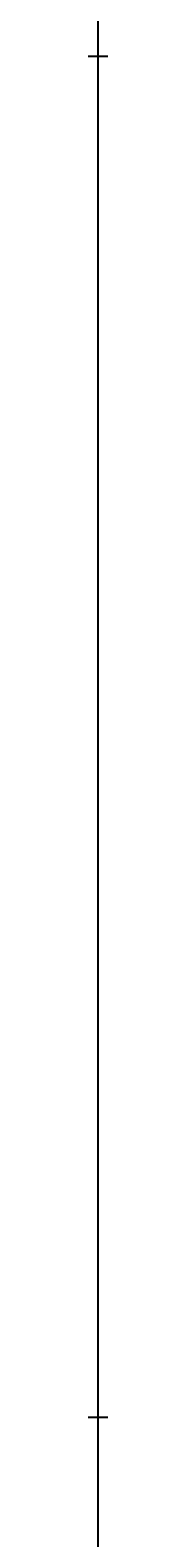
# Model space of a CAD drawing. Units: inches. Extents: x 35362 to 73946, y 43607 to 67532.
# Tile 34 of 134: x 48373 to 48373, y 46091 to 46564. Entities that reach past the tile are written whole.
import ezdxf

# ---------------------------------------------------------------- set-up
doc = ezdxf.new("R2010")
doc.units = ezdxf.units.IN
doc.header["$MEASUREMENT"] = 0
doc.layers.add('A-ANNO-DIMS', color=2, linetype='Continuous', lineweight=18)
doc.styles.get("Standard").update_dxf_attribs({"font": 'arial.ttf'})
doc.dimstyles.get("Standard").update_dxf_attribs({"dimtxt": 0.18, "dimasz": 0.18, "dimexe": 0.18, "dimexo": 0.0625, "dimgap": 0.09, "dimtad": 0, "dimtih": 1, "dimtoh": 1, "dimdec": 4, "dimzin": 0, "dimdsep": 46, "dimtxsty": 'Standard', "dimcen": 0.09, "dimadec": 0, "dimazin": 0, "dimtfac": 1, "dimtdec": 4, "dimtofl": 0, "dimtmove": 0, "dimatfit": 3, "dimfxl": 1, "dimtolj": 1, "dimtzin": 0, "dimarcsym": 0})

# ---------------------------------------------------------------- blocks, each defined once
blk = doc.blocks.new('*D5')
at = {"layer": 'A-ANNO-DIMS', "color": 0, "lineweight": -2, "transparency": 16777216}
for p, q in [((37121.95, 46919.32), (37121.95, 43606.68)), ((69871.5, 45449.83), (69871.5, 43606.68)), ((37122.13, 43606.86), (53496.29, 43606.86)), ((69871.32, 43606.86), (53497.15, 43606.86))]:
    blk.add_line(p, q, dxfattribs=at)
at = {"layer": 'A-ANNO-DIMS', "color": 0, "transparency": 16777216}
for points in [[(37122.13, 43606.89), (37122.13, 43606.83), (37121.95, 43606.86)], [(69871.32, 43606.89), (69871.32, 43606.83), (69871.5, 43606.86)]]:
    blk.add_solid(points, dxfattribs=at)
at = {"layer": 'Defpoints', "color": 0, "transparency": 16777216}
for p in [(37121.95, 46919.38), (69871.5, 45449.89), (69871.5, 43606.86)]:
    blk.add_point(p, dxfattribs=at)
at = {"layer": 'A-ANNO-DIMS', "color": 0, "transparency": 16777216, "insert": (53496.72, 43606.86), "char_height": 0.18, "attachment_point": 5}
blk.add_mtext('\\A1;32750', dxfattribs=at)
blk = doc.blocks.new('*D11')
at = {"layer": 'A-ANNO-DIMS', "color": 0, "lineweight": -2, "transparency": 16777216}
for p, q in [((47978.66, 56028.77), (47978.66, 43606.68)), ((53109.76, 56028.77), (53109.76, 43606.68)), ((47978.84, 43606.86), (50543.87, 43606.86)), ((53109.58, 43606.86), (50544.55, 43606.86))]:
    blk.add_line(p, q, dxfattribs=at)
at = {"layer": 'A-ANNO-DIMS', "color": 0, "transparency": 16777216}
for points in [[(47978.84, 43606.89), (47978.84, 43606.83), (47978.66, 43606.86)], [(53109.58, 43606.89), (53109.58, 43606.83), (53109.76, 43606.86)]]:
    blk.add_solid(points, dxfattribs=at)
at = {"layer": 'Defpoints', "color": 0, "transparency": 16777216}
for p in [(47978.66, 56028.84), (53109.76, 56028.84), (53109.76, 43606.86)]:
    blk.add_point(p, dxfattribs=at)
at = {"layer": 'A-ANNO-DIMS', "color": 0, "transparency": 16777216, "insert": (50544.21, 43606.86), "char_height": 0.18, "attachment_point": 5}
blk.add_mtext('\\A1;5131', dxfattribs=at)
blk = doc.blocks.new('*D13')
at = {"layer": 'A-ANNO-DIMS', "color": 0, "lineweight": -2, "transparency": 16777216}
for p, q in [((48373.49, 51694.02), (48373.49, 43606.68)), ((51029.04, 51694.02), (51029.04, 43606.68)), ((48373.67, 43606.86), (49700.8, 43606.86)), ((51028.86, 43606.86), (49701.73, 43606.86))]:
    blk.add_line(p, q, dxfattribs=at)
at = {"layer": 'A-ANNO-DIMS', "color": 0, "transparency": 16777216}
for points in [[(48373.67, 43606.89), (48373.67, 43606.83), (48373.49, 43606.86)], [(51028.86, 43606.89), (51028.86, 43606.83), (51029.04, 43606.86)]]:
    blk.add_solid(points, dxfattribs=at)
at = {"layer": 'Defpoints', "color": 0, "transparency": 16777216}
for p in [(48373.49, 51694.09), (51029.04, 51694.09), (51029.04, 43606.86)]:
    blk.add_point(p, dxfattribs=at)
at = {"layer": 'A-ANNO-DIMS', "color": 0, "transparency": 16777216, "insert": (49701.27, 43606.86), "char_height": 0.18, "attachment_point": 5}
blk.add_mtext('\\A1;2655.6', dxfattribs=at)
blk = doc.blocks.new('*D27')
at = {"layer": 'A-ANNO-DIMS', "color": 0, "lineweight": -2, "transparency": 16777216}
for p, q in [((47978.66, 56028.77), (47978.66, 43606.68)), ((48373.49, 53428.96), (48373.49, 43606.68)), ((47978.84, 43606.86), (48175.68, 43606.86)), ((48373.31, 43606.86), (48176.47, 43606.86))]:
    blk.add_line(p, q, dxfattribs=at)
at = {"layer": 'A-ANNO-DIMS', "color": 0, "transparency": 16777216}
for points in [[(47978.84, 43606.89), (47978.84, 43606.83), (47978.66, 43606.86)], [(48373.31, 43606.89), (48373.31, 43606.83), (48373.49, 43606.86)]]:
    blk.add_solid(points, dxfattribs=at)
at = {"layer": 'Defpoints', "color": 0, "transparency": 16777216}
for p in [(47978.66, 56028.84), (48373.49, 53429.02), (48373.49, 43606.86)]:
    blk.add_point(p, dxfattribs=at)
at = {"layer": 'A-ANNO-DIMS', "color": 0, "transparency": 16777216, "insert": (48176.08, 43606.86), "char_height": 0.18, "attachment_point": 5}
blk.add_mtext('\\A1;394.8', dxfattribs=at)
blk = doc.blocks.new('*D67')
at = {"layer": 'A-ANNO-DIMS', "color": 0, "lineweight": -2, "transparency": 16777216}
for p, q in [((56873.54, 53351.53), (35361.77, 53351.53)), ((35361.95, 53351.35), (35361.95, 49400.89)), ((35361.95, 45450.07), (35361.95, 49400.53)), ((53793.58, 45449.89), (35361.77, 45449.89))]:
    blk.add_line(p, q, dxfattribs=at)
at = {"layer": 'A-ANNO-DIMS', "color": 0, "transparency": 16777216}
for points in [[(35361.92, 53351.35), (35361.98, 53351.35), (35361.95, 53351.53)], [(35361.92, 45450.07), (35361.98, 45450.07), (35361.95, 45449.89)]]:
    blk.add_solid(points, dxfattribs=at)
at = {"layer": 'Defpoints', "color": 0, "transparency": 16777216}
for p in [(35361.95, 53351.53), (56873.6, 53351.53), (53793.64, 45449.89)]:
    blk.add_point(p, dxfattribs=at)
at = {"layer": 'A-ANNO-DIMS', "color": 0, "transparency": 16777216, "insert": (35361.95, 49400.71), "char_height": 0.18, "attachment_point": 5}
blk.add_mtext('\\A1;7901.6', dxfattribs=at)
blk = doc.blocks.new('*D76')
at = {"layer": 'A-ANNO-DIMS', "color": 0, "lineweight": -2, "transparency": 16777216}
for p, q in [((54052.84, 46555.29), (35361.77, 46555.29)), ((35361.95, 46555.11), (35361.95, 46342.27)), ((35361.95, 46129.06), (35361.95, 46341.9)), ((53793.58, 46128.88), (35361.77, 46128.88))]:
    blk.add_line(p, q, dxfattribs=at)
at = {"layer": 'A-ANNO-DIMS', "color": 0, "transparency": 16777216}
for points in [[(35361.92, 46555.11), (35361.98, 46555.11), (35361.95, 46555.29)], [(35361.92, 46129.06), (35361.98, 46129.06), (35361.95, 46128.88)]]:
    blk.add_solid(points, dxfattribs=at)
at = {"layer": 'Defpoints', "color": 0, "transparency": 16777216}
for p in [(35361.95, 46555.29), (54052.9, 46555.29), (53793.64, 46128.88)]:
    blk.add_point(p, dxfattribs=at)
at = {"layer": 'A-ANNO-DIMS', "color": 0, "transparency": 16777216, "insert": (35361.95, 46342.09), "char_height": 0.18, "attachment_point": 5}
blk.add_mtext('\\A1;426.4', dxfattribs=at)
blk = doc.blocks.new('*D90')
at = {"layer": 'A-ANNO-DIMS', "color": 0, "lineweight": -2, "transparency": 16777216}
for p, q in [((53707.72, 47291.29), (35361.77, 47291.29)), ((35361.95, 47291.11), (35361.95, 46710.26)), ((35361.95, 46129.06), (35361.95, 46709.9)), ((53793.58, 46128.88), (35361.77, 46128.88))]:
    blk.add_line(p, q, dxfattribs=at)
at = {"layer": 'A-ANNO-DIMS', "color": 0, "transparency": 16777216}
for points in [[(35361.92, 47291.11), (35361.98, 47291.11), (35361.95, 47291.29)], [(35361.92, 46129.06), (35361.98, 46129.06), (35361.95, 46128.88)]]:
    blk.add_solid(points, dxfattribs=at)
at = {"layer": 'Defpoints', "color": 0, "transparency": 16777216}
for p in [(53707.78, 47291.29), (35361.95, 46128.88), (53793.64, 46128.88)]:
    blk.add_point(p, dxfattribs=at)
at = {"layer": 'A-ANNO-DIMS', "color": 0, "transparency": 16777216, "insert": (35361.95, 46710.08), "char_height": 0.18, "attachment_point": 5}
blk.add_mtext('\\A1;1162.4', dxfattribs=at)

msp = doc.modelspace()

# ---------------------------------------------------------------- dimensions: what is measured, and where the dimension line sits
at = {"layer": 'A-ANNO-DIMS'}
for base, p1, p2, override, picture, middle in [((53109.76, 43606.859), (47978.665, 56028.836), (53109.76, 56028.836), {"dimdec": 0, "dimlfac": 1, "dimrnd": 0, "dimzin": 0, "dimdsep": 46, "dimlunit": 2}, '*D11', (50544.212, 43606.859)), ((48373.492, 43606.859), (47978.665, 56028.836), (48373.492, 53429.019), {"dimdec": 1, "dimlfac": 1, "dimrnd": 0, "dimzin": 0, "dimdsep": 46, "dimlunit": 2}, '*D27', (48176.078, 43606.859)), ((51029.043, 43606.859), (48373.492, 51694.087), (51029.043, 51694.087), {"dimdec": 1, "dimlfac": 1, "dimrnd": 0, "dimzin": 0, "dimdsep": 46, "dimlunit": 2}, '*D13', (49701.267, 43606.859)), ((69871.496, 43606.859), (37121.949, 46919.381), (69871.496, 45449.894), {"dimdec": 0, "dimlfac": 1, "dimrnd": 0, "dimzin": 0, "dimdsep": 46, "dimlunit": 2}, '*D5', (53496.723, 43606.859))]:
    dim = msp.add_linear_dim(base=base, p1=p1, p2=p2, dimstyle='Standard', override=override, dxfattribs=at)
    dim.commit()
    dim.dimension.update_dxf_attribs({"geometry": picture, "text_midpoint": middle})
for base, p1, p2, picture, middle in [((35361.949, 53351.529), (53793.638, 45449.894), (56873.602, 53351.529), '*D67', (35361.949, 49400.712)), ((35361.949, 46128.878), (53707.781, 47291.285), (53793.638, 46128.878), '*D90', (35361.949, 46710.081)), ((35361.949, 46555.293), (53793.638, 46128.878), (54052.899, 46555.293), '*D76', (35361.949, 46342.086))]:
    dim = msp.add_linear_dim(base=base, p1=p1, p2=p2, angle=90, dimstyle='Standard', override={"dimdec": 1, "dimlfac": 1, "dimrnd": 0, "dimzin": 0, "dimdsep": 46, "dimlunit": 2}, dxfattribs=at)
    dim.commit()
    dim.dimension.update_dxf_attribs({"geometry": picture, "text_midpoint": middle})

doc.saveas('drawing.dxf')
